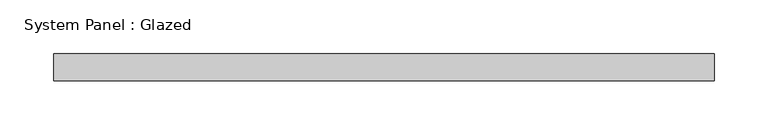
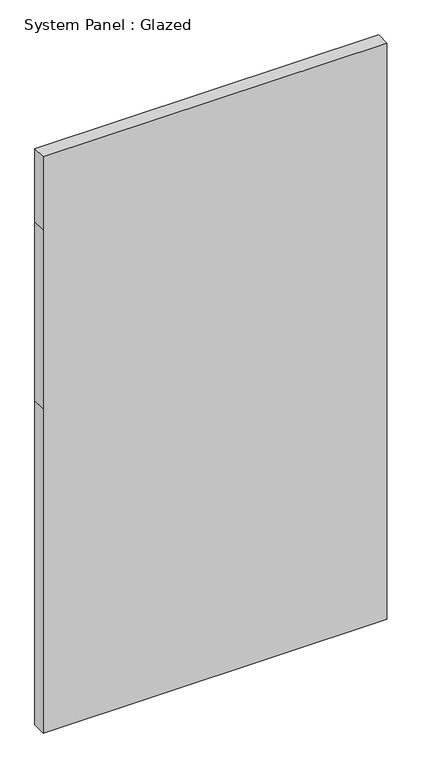
"""IFC4 building model written with IfcOpenShell, lengths in millimetres: plate geometry, System Panel : Glazed."""

from ifc_helpers import new_model, si_unit, frame, origin, place, context, project, spatial, polyline, outline, extrude, source, transform, mapped, element, save


def system_panel_glazed_68735acb(model_context):
    return source(origin(), model_context, "Body", "SweptSolid", [
        extrude(outline(polyline([(0.0, -307.975), (0.0, 307.975), (614.4496655, 307.975), (953.4244982, 307.975), (1091.1619146, 307.975), (1091.1619146, -307.975), (953.4244982, -307.975), (614.4496655, -307.975), (0.0, -307.975)])), frame((0.0, 19.05, 0.0), z_axis=(0.0, 1.0, 0.0), x_axis=(0.0, 0.0, 1.0)), (0.0, 0.0, 1.0), 25.4),
    ])


if __name__ == "__main__":
    model = new_model("IFC4")
    model_context = context("Model", 3, world=origin())
    ifc_project = project(units=[si_unit("LENGTHUNIT", "METRE", prefix="MILLI")], contexts=[model_context])
    site = spatial("IfcSite", under=ifc_project)
    building = spatial("IfcBuilding", under=site)
    placement = place(None, origin())
    system_panel_glazed_shape = system_panel_glazed_68735acb(model_context)
    element("IfcPlate", 1, ObjectType="System Panel : Glazed", at=placement, inside=building, context=model_context, shape_type="MappedRepresentation", body=[
        mapped(system_panel_glazed_shape, transform((0.0, 0.0, 0.0), x_axis=(1.0, 0.0, 0.0), y_axis=(0.0, 1.0, 0.0), z_axis=(0.0, 0.0, 1.0))),
    ])
    save(model, "model.ifc")

# Revit data of these elements
# Type "System Panel : Glazed"
#   Construction Type Id = "GSP4R"
#   Analytic Construction = "1/8 in Pilkington single glazing"
#   Visual Light Transmittance = 0.9
#   Solar Heat Gain Coefficient = 0.86
#   Heat Transfer Coefficient (U) = 1.18115 BTU/(h·ft²·°F)
#   Define Thermal Properties by = 1
# Element 1 (IfcPlate, "System Panel : Glazed")
#   Materials on its faces: "Glass"
# Materials
#   "Glass": class "Glass", colour RGB 0 128 192, transparency 0.75, Description = "Soda Lime Glass", Cost = 0
